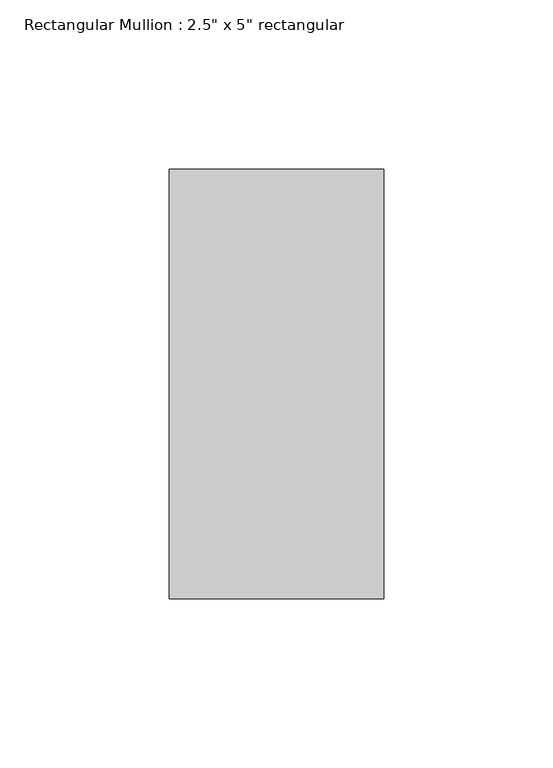
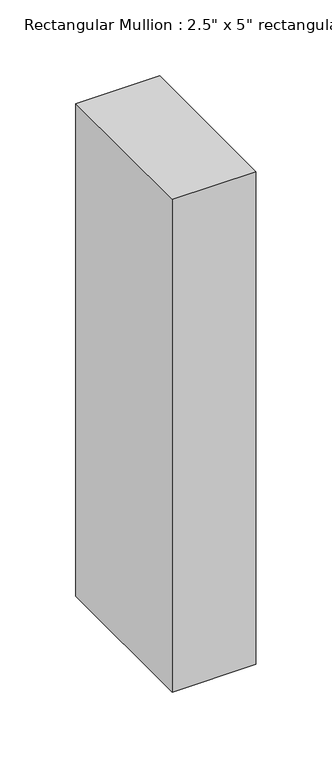
"""IFC4 building model written with IfcOpenShell, lengths in millimetres: member geometry."""

from ifc_helpers import new_model, si_unit, frame, origin, place, context, project, spatial, polyline, outline, extrude, source, transform, mapped, element, save


def member_1c9dfce7(model_context):
    return source(origin(), model_context, "Body", "SweptSolid", [
        extrude(outline(polyline([(0.0, 63.5), (0.0, -63.5), (-63.5, -63.5), (-63.5, 63.5), (0.0, 63.5)])), frame((0.0, 0.0, -395.8166667), z_axis=(0.0, 0.0, 1.0), x_axis=(1.0, 0.0, 0.0)), (0.0, 0.0, 1.0), 395.8166667),
    ])


if __name__ == "__main__":
    model = new_model("IFC4")
    model_context = context("Model", 3, world=origin())
    ifc_project = project(units=[si_unit("LENGTHUNIT", "METRE", prefix="MILLI")], contexts=[model_context])
    site = spatial("IfcSite", under=ifc_project)
    building = spatial("IfcBuilding", under=site)
    placement = place(None, origin())
    member_shape = member_1c9dfce7(model_context)
    element("IfcMember", 1, ObjectType="Rectangular Mullion : 2.5\" x 5\" rectangular", at=placement, inside=building, context=model_context, shape_type="MappedRepresentation", body=[
        mapped(member_shape, transform((0.0, 0.0, 0.0), x_axis=(1.0, 0.0, 0.0), y_axis=(0.0, 1.0, 0.0), z_axis=(0.0, 0.0, 1.0))),
    ])
    save(model, "model.ifc")

# Revit data of these elements
# Type "Rectangular Mullion : 2.5\" x 5\" rectangular"
#   built-in parameter 1007304 = 0.416667 (stored number, unit not read)
#   built-in parameter 1007301 = 0.104167 (stored number, unit not read)
#   built-in parameter 1007300 = 0.104167 (stored number, unit not read)
